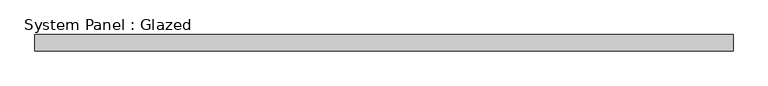
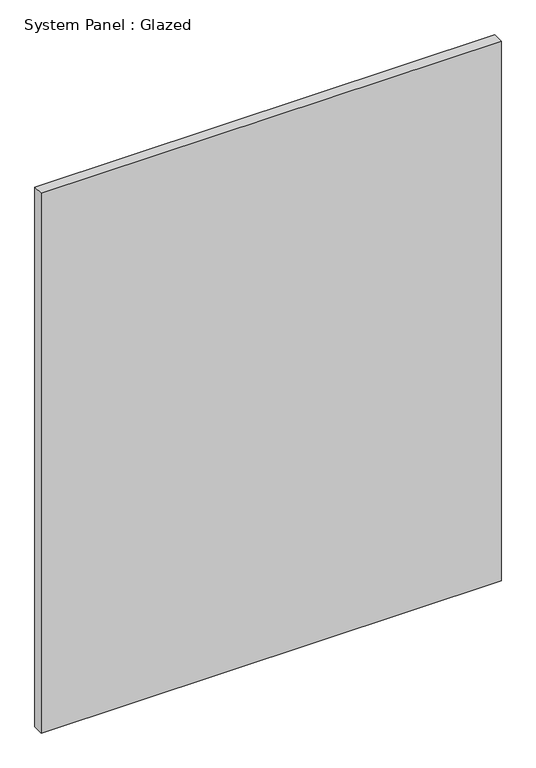
"""IFC4 building model written with IfcOpenShell, lengths in millimetres: plate geometry, System Panel : Glazed."""

from ifc_helpers import new_model, si_unit, origin, origin_with_axes, place, context, project, spatial, polyline, outline, extrude, source, transform, mapped, element, save


def system_panel_glazed_abc17199(model_context):
    return source(origin(), model_context, "Body", "SweptSolid", [
        extrude(outline(polyline([(535.0, 24.5), (-535.0, 24.5), (-535.0, 49.5), (535.0, 49.5), (535.0, 24.5)])), origin_with_axes(), (0.0, 0.0, 1.0), 1327.5),
    ])


if __name__ == "__main__":
    model = new_model("IFC4")
    model_context = context("Model", 3, world=origin())
    ifc_project = project(units=[si_unit("LENGTHUNIT", "METRE", prefix="MILLI")], contexts=[model_context])
    site = spatial("IfcSite", under=ifc_project)
    building = spatial("IfcBuilding", under=site)
    placement = place(None, origin())
    system_panel_glazed_shape = system_panel_glazed_abc17199(model_context)
    element("IfcPlate", 1, ObjectType="System Panel : Glazed", at=placement, inside=building, context=model_context, shape_type="MappedRepresentation", body=[
        mapped(system_panel_glazed_shape, transform((0.0, 0.0, 0.0), x_axis=(1.0, 0.0, 0.0), y_axis=(0.0, 1.0, 0.0), z_axis=(0.0, 0.0, 1.0))),
    ])
    save(model, "model.ifc")

# Revit data of these elements
# Type "System Panel : Glazed"
#   Construction Type Id = "GSP4R"
#   Analytic Construction = "1/8 in Pilkington single glazing"
#   Visual Light Transmittance = 0.9
#   Solar Heat Gain Coefficient = 0.86
#   Heat Transfer Coefficient (U) = 6.7069 W/(m²·K)
#   Define Thermal Properties by = 1
# Element 1 (IfcPlate, "System Panel : Glazed")
#   Materials on its faces: "Glass"
# Materials
#   "Glass": class "Glass", colour RGB 245 245 243, transparency 1, Description = "Soda Lime Glass", Cost = 0
